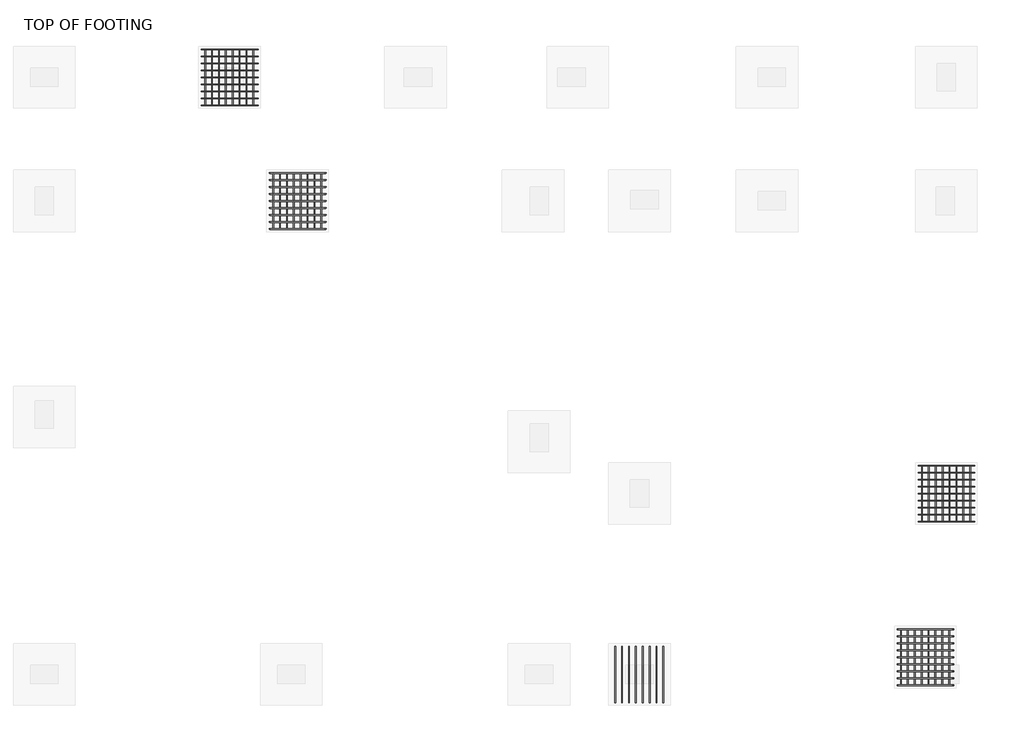
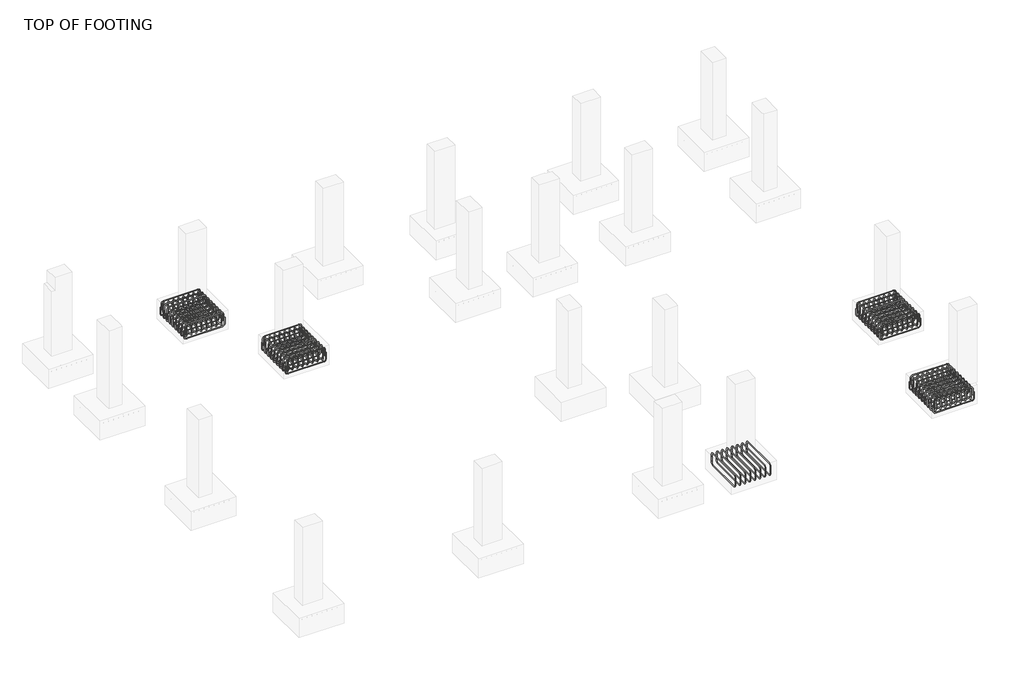
# One storey, part 6 of 20: 18 reinforcing bars.
"""IFC4 building model written with IfcOpenShell, lengths in millimetres."""

from ifc_helpers import new_model, si_unit, point, frame, origin, place, context, project, spatial, polyline, circle_curve, trimmed, segment, composite_curve, source, transform, mapped, element, save
from ifc_brep_helpers import swept_disk

model = new_model("IFC4")

# Units and contexts
model_context = context("Model", 3, world=origin())
ifc_project = project(units=[si_unit("LENGTHUNIT", "METRE", prefix="MILLI")], contexts=[model_context])

# Site, building, storey
site = spatial("IfcSite", under=ifc_project)
building = spatial("IfcBuilding", under=site)
storey = spatial("IfcBuildingStorey", under=building, Name="TOP OF FOOTING", Elevation=-1828.8)

# Reinforcing bars
placement = place(None, origin())
reinforcing_bar_shape = source(origin(), model_context, "Body", "SolidModel", [
    swept_disk(composite_curve([segment(polyline([(8189.02094, -18968.8804373, -2086.1951968), (8189.02094, -18968.8804373, -1938.8951968)]), True, "CONTINUOUS"), segment(trimmed(circle_curve(frame((8189.02094, -19015.2304373, -1938.8951968), z_axis=(1.0, 0.0, 0.0), x_axis=(0.0, 46.35000000000218, 0.0)), 46.35), [point((8189.02094, -18968.8804373, -1938.8951968))], [point((8189.02094, -19015.2304373, -1892.5451968))], True, "CARTESIAN"), True, "CONTINUOUS"), segment(polyline([(8189.02094, -19015.2304373, -1892.5451968), (8189.02094, -19829.8304373, -1892.5451968)]), True, "CONTINUOUS"), segment(trimmed(circle_curve(frame((8189.02094, -19829.8304373, -1938.8951968), z_axis=(1.0, 0.0, 0.0), x_axis=(0.0, 0.0, 46.34999999999991)), 46.35), [point((8189.02094, -19829.8304373, -1892.5451968))], [point((8189.02094, -19876.1804373, -1938.8951968))], True, "CARTESIAN"), True, "CONTINUOUS"), segment(polyline([(8189.02094, -19876.1804373, -1938.8951968), (8189.02094, -19876.1804373, -2086.1951968)]), True, "CONTINUOUS")], self_intersect=False), 6.35),
])
element("IfcReinforcingBar", 1, at=placement, inside=storey, context=model_context, shape_type="MappedRepresentation", body=[
    mapped(reinforcing_bar_shape, transform((0.0, 0.0, 0.0), x_axis=(1.0, 0.0, 0.0), y_axis=(0.0, 1.0, 0.0), z_axis=(0.0, 0.0, 1.0))),
    mapped(reinforcing_bar_shape, transform((-111.2862402, 0.0, 0.0), x_axis=(1.0, 0.0, 0.0), y_axis=(0.0, 1.0, 0.0), z_axis=(0.0, 0.0, 1.0))),
    mapped(reinforcing_bar_shape, transform((-222.5724804, 0.0, 0.0), x_axis=(1.0, 0.0, 0.0), y_axis=(0.0, 1.0, 0.0), z_axis=(0.0, 0.0, 1.0))),
    mapped(reinforcing_bar_shape, transform((-333.8587205, 0.0, 0.0), x_axis=(1.0, 0.0, 0.0), y_axis=(0.0, 1.0, 0.0), z_axis=(0.0, 0.0, 1.0))),
    mapped(reinforcing_bar_shape, transform((-445.1449607, 0.0, 0.0), x_axis=(1.0, 0.0, 0.0), y_axis=(0.0, 1.0, 0.0), z_axis=(0.0, 0.0, 1.0))),
    mapped(reinforcing_bar_shape, transform((-556.4312009, 0.0, 0.0), x_axis=(1.0, 0.0, 0.0), y_axis=(0.0, 1.0, 0.0), z_axis=(0.0, 0.0, 1.0))),
    mapped(reinforcing_bar_shape, transform((-667.7174411, 0.0, 0.0), x_axis=(1.0, 0.0, 0.0), y_axis=(0.0, 1.0, 0.0), z_axis=(0.0, 0.0, 1.0))),
    mapped(reinforcing_bar_shape, transform((-779.0036813, 0.0, 0.0), x_axis=(1.0, 0.0, 0.0), y_axis=(0.0, 1.0, 0.0), z_axis=(0.0, 0.0, 1.0))),
])
reinforcing_bar_2_shape = source(origin(), model_context, "Body", "SolidModel", [
    swept_disk(composite_curve([segment(polyline([(7410.0172587, -18968.8804373, -1979.1645013), (7410.0172587, -18968.8804373, -2126.4645013)]), True, "CONTINUOUS"), segment(trimmed(circle_curve(frame((7410.0172587, -19015.2304373, -2126.4645013), z_axis=(-1.0, 0.0, 0.0), x_axis=(0.0, 46.35000000000218, 0.0)), 46.35), [point((7410.0172587, -18968.8804373, -2126.4645013))], [point((7410.0172587, -19015.2304373, -2172.8145013))], True, "CARTESIAN"), True, "CONTINUOUS"), segment(polyline([(7410.0172587, -19015.2304373, -2172.8145013), (7410.0172587, -19829.8304373, -2172.8145013)]), True, "CONTINUOUS"), segment(trimmed(circle_curve(frame((7410.0172587, -19829.8304373, -2126.4645013), z_axis=(-1.0, 0.0, 0.0), x_axis=(0.0, 0.0, -46.34999999999991)), 46.35), [point((7410.0172587, -19829.8304373, -2172.8145013))], [point((7410.0172587, -19876.1804373, -2126.4645013))], True, "CARTESIAN"), True, "CONTINUOUS"), segment(polyline([(7410.0172587, -19876.1804373, -2126.4645013), (7410.0172587, -19876.1804373, -1979.1645013)]), True, "CONTINUOUS")], self_intersect=False), 6.35),
])
element("IfcReinforcingBar", 2, at=placement, inside=storey, context=model_context, shape_type="MappedRepresentation", body=[
    mapped(reinforcing_bar_2_shape, transform((0.0, 0.0, 0.0), x_axis=(1.0, 0.0, 0.0), y_axis=(0.0, 1.0, 0.0), z_axis=(0.0, 0.0, 1.0))),
    mapped(reinforcing_bar_2_shape, transform((111.2862402, 0.0, 0.0), x_axis=(1.0, 0.0, 0.0), y_axis=(0.0, 1.0, 0.0), z_axis=(0.0, 0.0, 1.0))),
    mapped(reinforcing_bar_2_shape, transform((222.5724804, 0.0, 0.0), x_axis=(1.0, 0.0, 0.0), y_axis=(0.0, 1.0, 0.0), z_axis=(0.0, 0.0, 1.0))),
    mapped(reinforcing_bar_2_shape, transform((333.8587205, 0.0, 0.0), x_axis=(1.0, 0.0, 0.0), y_axis=(0.0, 1.0, 0.0), z_axis=(0.0, 0.0, 1.0))),
    mapped(reinforcing_bar_2_shape, transform((445.1449607, 0.0, 0.0), x_axis=(1.0, 0.0, 0.0), y_axis=(0.0, 1.0, 0.0), z_axis=(0.0, 0.0, 1.0))),
    mapped(reinforcing_bar_2_shape, transform((556.4312009, 0.0, 0.0), x_axis=(1.0, 0.0, 0.0), y_axis=(0.0, 1.0, 0.0), z_axis=(0.0, 0.0, 1.0))),
    mapped(reinforcing_bar_2_shape, transform((667.7174411, 0.0, 0.0), x_axis=(1.0, 0.0, 0.0), y_axis=(0.0, 1.0, 0.0), z_axis=(0.0, 0.0, 1.0))),
    mapped(reinforcing_bar_2_shape, transform((779.0036813, 0.0, 0.0), x_axis=(1.0, 0.0, 0.0), y_axis=(0.0, 1.0, 0.0), z_axis=(0.0, 0.0, 1.0))),
])
reinforcing_bar_3_shape = source(origin(), model_context, "Body", "SolidModel", [
    swept_disk(composite_curve([segment(polyline([(12882.7663908, -18688.8804373, -2006.6587682), (12882.7663908, -18688.8804373, -2153.9587682)]), True, "CONTINUOUS"), segment(trimmed(circle_curve(frame((12836.4163908, -18688.8804373, -2153.9587682), z_axis=(0.0, 1.0, 0.0), x_axis=(46.350000000000364, 0.0, 0.0)), 46.35), [point((12882.7663908, -18688.8804373, -2153.9587682))], [point((12836.4163908, -18688.8804373, -2200.3087682))], True, "CARTESIAN"), True, "CONTINUOUS"), segment(polyline([(12836.4163908, -18688.8804373, -2200.3087682), (12021.8163908, -18688.8804373, -2200.3087682)]), True, "CONTINUOUS"), segment(trimmed(circle_curve(frame((12021.8163908, -18688.8804373, -2153.9587682), z_axis=(0.0, 1.0, 0.0), x_axis=(0.0, 0.0, -46.34999999999991)), 46.35), [point((12021.8163908, -18688.8804373, -2200.3087682))], [point((11975.4663908, -18688.8804373, -2153.9587682))], True, "CARTESIAN"), True, "CONTINUOUS"), segment(polyline([(11975.4663908, -18688.8804373, -2153.9587682), (11975.4663908, -18688.8804373, -2006.6587682)]), True, "CONTINUOUS")], self_intersect=False), 6.35),
])
element("IfcReinforcingBar", 3, at=placement, inside=storey, context=model_context, shape_type="MappedRepresentation", body=[
    mapped(reinforcing_bar_3_shape, transform((0.0, 0.0, 0.0), x_axis=(1.0, 0.0, 0.0), y_axis=(0.0, 1.0, 0.0), z_axis=(0.0, 0.0, 1.0))),
    mapped(reinforcing_bar_3_shape, transform((0.0, -113.4125, 0.0), x_axis=(1.0, 0.0, 0.0), y_axis=(0.0, 1.0, 0.0), z_axis=(0.0, 0.0, 1.0))),
    mapped(reinforcing_bar_3_shape, transform((0.0, -226.825, 0.0), x_axis=(1.0, 0.0, 0.0), y_axis=(0.0, 1.0, 0.0), z_axis=(0.0, 0.0, 1.0))),
    mapped(reinforcing_bar_3_shape, transform((0.0, -340.2375, 0.0), x_axis=(1.0, 0.0, 0.0), y_axis=(0.0, 1.0, 0.0), z_axis=(0.0, 0.0, 1.0))),
    mapped(reinforcing_bar_3_shape, transform((0.0, -453.65, 0.0), x_axis=(1.0, 0.0, 0.0), y_axis=(0.0, 1.0, 0.0), z_axis=(0.0, 0.0, 1.0))),
    mapped(reinforcing_bar_3_shape, transform((0.0, -567.0625, 0.0), x_axis=(1.0, 0.0, 0.0), y_axis=(0.0, 1.0, 0.0), z_axis=(0.0, 0.0, 1.0))),
    mapped(reinforcing_bar_3_shape, transform((0.0, -680.475, 0.0), x_axis=(1.0, 0.0, 0.0), y_axis=(0.0, 1.0, 0.0), z_axis=(0.0, 0.0, 1.0))),
    mapped(reinforcing_bar_3_shape, transform((0.0, -793.8875, 0.0), x_axis=(1.0, 0.0, 0.0), y_axis=(0.0, 1.0, 0.0), z_axis=(0.0, 0.0, 1.0))),
    mapped(reinforcing_bar_3_shape, transform((0.0, -907.3, 0.0), x_axis=(1.0, 0.0, 0.0), y_axis=(0.0, 1.0, 0.0), z_axis=(0.0, 0.0, 1.0))),
])
reinforcing_bar_4_shape = source(origin(), model_context, "Body", "SolidModel", [
    swept_disk(composite_curve([segment(polyline([(11994.9405021, -18688.8804373, -2068.8), (11994.9405021, -18688.8804373, -1921.5)]), True, "CONTINUOUS"), segment(trimmed(circle_curve(frame((12041.2905021, -18688.8804373, -1921.5), z_axis=(0.0, 1.0, 0.0), x_axis=(-46.350000000000364, 0.0, 0.0)), 46.35), [point((11994.9405021, -18688.8804373, -1921.5))], [point((12041.2905021, -18688.8804373, -1875.15))], True, "CARTESIAN"), True, "CONTINUOUS"), segment(polyline([(12041.2905021, -18688.8804373, -1875.15), (12810.7539017, -18688.8804373, -1875.15)]), True, "CONTINUOUS"), segment(trimmed(circle_curve(frame((12810.7539017, -18688.8804373, -1921.5), z_axis=(0.0, 1.0, 0.0), x_axis=(0.0, 0.0, 46.34999999999991)), 46.35), [point((12810.7539017, -18688.8804373, -1875.15))], [point((12857.1039017, -18688.8804373, -1921.5))], True, "CARTESIAN"), True, "CONTINUOUS"), segment(polyline([(12857.1039017, -18688.8804373, -1921.5), (12857.1039017, -18688.8804373, -2068.8)]), True, "CONTINUOUS")], self_intersect=False), 6.35),
])
element("IfcReinforcingBar", 4, at=placement, inside=storey, context=model_context, shape_type="MappedRepresentation", body=[
    mapped(reinforcing_bar_4_shape, transform((0.0, 0.0, 0.0), x_axis=(1.0, 0.0, 0.0), y_axis=(0.0, 1.0, 0.0), z_axis=(0.0, 0.0, 1.0))),
    mapped(reinforcing_bar_4_shape, transform((0.0, -113.4125, 0.0), x_axis=(1.0, 0.0, 0.0), y_axis=(0.0, 1.0, 0.0), z_axis=(0.0, 0.0, 1.0))),
    mapped(reinforcing_bar_4_shape, transform((0.0, -226.825, 0.0), x_axis=(1.0, 0.0, 0.0), y_axis=(0.0, 1.0, 0.0), z_axis=(0.0, 0.0, 1.0))),
    mapped(reinforcing_bar_4_shape, transform((0.0, -340.2375, 0.0), x_axis=(1.0, 0.0, 0.0), y_axis=(0.0, 1.0, 0.0), z_axis=(0.0, 0.0, 1.0))),
    mapped(reinforcing_bar_4_shape, transform((0.0, -453.65, 0.0), x_axis=(1.0, 0.0, 0.0), y_axis=(0.0, 1.0, 0.0), z_axis=(0.0, 0.0, 1.0))),
    mapped(reinforcing_bar_4_shape, transform((0.0, -567.0625, 0.0), x_axis=(1.0, 0.0, 0.0), y_axis=(0.0, 1.0, 0.0), z_axis=(0.0, 0.0, 1.0))),
    mapped(reinforcing_bar_4_shape, transform((0.0, -680.475, 0.0), x_axis=(1.0, 0.0, 0.0), y_axis=(0.0, 1.0, 0.0), z_axis=(0.0, 0.0, 1.0))),
    mapped(reinforcing_bar_4_shape, transform((0.0, -793.8875, 0.0), x_axis=(1.0, 0.0, 0.0), y_axis=(0.0, 1.0, 0.0), z_axis=(0.0, 0.0, 1.0))),
    mapped(reinforcing_bar_4_shape, transform((0.0, -907.3, 0.0), x_axis=(1.0, 0.0, 0.0), y_axis=(0.0, 1.0, 0.0), z_axis=(0.0, 0.0, 1.0))),
])
reinforcing_bar_5_shape = source(origin(), model_context, "Body", "SolidModel", [
    swept_disk(composite_curve([segment(polyline([(12811.2694294, -18688.8804373, -2086.1951968), (12811.2694294, -18688.8804373, -1938.8951968)]), True, "CONTINUOUS"), segment(trimmed(circle_curve(frame((12811.2694294, -18735.2304373, -1938.8951968), z_axis=(1.0, 0.0, 0.0), x_axis=(0.0, 46.35000000000218, 0.0)), 46.35), [point((12811.2694294, -18688.8804373, -1938.8951968))], [point((12811.2694294, -18735.2304373, -1892.5451968))], True, "CARTESIAN"), True, "CONTINUOUS"), segment(polyline([(12811.2694294, -18735.2304373, -1892.5451968), (12811.2694294, -19549.8304373, -1892.5451968)]), True, "CONTINUOUS"), segment(trimmed(circle_curve(frame((12811.2694294, -19549.8304373, -1938.8951968), z_axis=(1.0, 0.0, 0.0), x_axis=(0.0, 0.0, 46.34999999999991)), 46.35), [point((12811.2694294, -19549.8304373, -1892.5451968))], [point((12811.2694294, -19596.1804373, -1938.8951968))], True, "CARTESIAN"), True, "CONTINUOUS"), segment(polyline([(12811.2694294, -19596.1804373, -1938.8951968), (12811.2694294, -19596.1804373, -2086.1951968)]), True, "CONTINUOUS")], self_intersect=False), 6.35),
])
element("IfcReinforcingBar", 5, at=placement, inside=storey, context=model_context, shape_type="MappedRepresentation", body=[
    mapped(reinforcing_bar_5_shape, transform((0.0, 0.0, 0.0), x_axis=(1.0, 0.0, 0.0), y_axis=(0.0, 1.0, 0.0), z_axis=(0.0, 0.0, 1.0))),
    mapped(reinforcing_bar_5_shape, transform((-111.2862402, 0.0, 0.0), x_axis=(1.0, 0.0, 0.0), y_axis=(0.0, 1.0, 0.0), z_axis=(0.0, 0.0, 1.0))),
    mapped(reinforcing_bar_5_shape, transform((-222.5724804, 0.0, 0.0), x_axis=(1.0, 0.0, 0.0), y_axis=(0.0, 1.0, 0.0), z_axis=(0.0, 0.0, 1.0))),
    mapped(reinforcing_bar_5_shape, transform((-333.8587205, 0.0, 0.0), x_axis=(1.0, 0.0, 0.0), y_axis=(0.0, 1.0, 0.0), z_axis=(0.0, 0.0, 1.0))),
    mapped(reinforcing_bar_5_shape, transform((-445.1449607, 0.0, 0.0), x_axis=(1.0, 0.0, 0.0), y_axis=(0.0, 1.0, 0.0), z_axis=(0.0, 0.0, 1.0))),
    mapped(reinforcing_bar_5_shape, transform((-556.4312009, 0.0, 0.0), x_axis=(1.0, 0.0, 0.0), y_axis=(0.0, 1.0, 0.0), z_axis=(0.0, 0.0, 1.0))),
    mapped(reinforcing_bar_5_shape, transform((-667.7174411, 0.0, 0.0), x_axis=(1.0, 0.0, 0.0), y_axis=(0.0, 1.0, 0.0), z_axis=(0.0, 0.0, 1.0))),
    mapped(reinforcing_bar_5_shape, transform((-779.0036813, 0.0, 0.0), x_axis=(1.0, 0.0, 0.0), y_axis=(0.0, 1.0, 0.0), z_axis=(0.0, 0.0, 1.0))),
])
reinforcing_bar_6_shape = source(origin(), model_context, "Body", "SolidModel", [
    swept_disk(composite_curve([segment(polyline([(12032.2657481, -18688.8804373, -1979.1645013), (12032.2657481, -18688.8804373, -2126.4645013)]), True, "CONTINUOUS"), segment(trimmed(circle_curve(frame((12032.2657481, -18735.2304373, -2126.4645013), z_axis=(-1.0, 0.0, 0.0), x_axis=(0.0, 46.35000000000218, 0.0)), 46.35), [point((12032.2657481, -18688.8804373, -2126.4645013))], [point((12032.2657481, -18735.2304373, -2172.8145013))], True, "CARTESIAN"), True, "CONTINUOUS"), segment(polyline([(12032.2657481, -18735.2304373, -2172.8145013), (12032.2657481, -19549.8304373, -2172.8145013)]), True, "CONTINUOUS"), segment(trimmed(circle_curve(frame((12032.2657481, -19549.8304373, -2126.4645013), z_axis=(-1.0, 0.0, 0.0), x_axis=(0.0, 0.0, -46.34999999999991)), 46.35), [point((12032.2657481, -19549.8304373, -2172.8145013))], [point((12032.2657481, -19596.1804373, -2126.4645013))], True, "CARTESIAN"), True, "CONTINUOUS"), segment(polyline([(12032.2657481, -19596.1804373, -2126.4645013), (12032.2657481, -19596.1804373, -1979.1645013)]), True, "CONTINUOUS")], self_intersect=False), 6.35),
])
element("IfcReinforcingBar", 6, at=placement, inside=storey, context=model_context, shape_type="MappedRepresentation", body=[
    mapped(reinforcing_bar_6_shape, transform((0.0, 0.0, 0.0), x_axis=(1.0, 0.0, 0.0), y_axis=(0.0, 1.0, 0.0), z_axis=(0.0, 0.0, 1.0))),
    mapped(reinforcing_bar_6_shape, transform((111.2862402, 0.0, 0.0), x_axis=(1.0, 0.0, 0.0), y_axis=(0.0, 1.0, 0.0), z_axis=(0.0, 0.0, 1.0))),
    mapped(reinforcing_bar_6_shape, transform((222.5724804, 0.0, 0.0), x_axis=(1.0, 0.0, 0.0), y_axis=(0.0, 1.0, 0.0), z_axis=(0.0, 0.0, 1.0))),
    mapped(reinforcing_bar_6_shape, transform((333.8587205, 0.0, 0.0), x_axis=(1.0, 0.0, 0.0), y_axis=(0.0, 1.0, 0.0), z_axis=(0.0, 0.0, 1.0))),
    mapped(reinforcing_bar_6_shape, transform((445.1449607, 0.0, 0.0), x_axis=(1.0, 0.0, 0.0), y_axis=(0.0, 1.0, 0.0), z_axis=(0.0, 0.0, 1.0))),
    mapped(reinforcing_bar_6_shape, transform((556.4312009, 0.0, 0.0), x_axis=(1.0, 0.0, 0.0), y_axis=(0.0, 1.0, 0.0), z_axis=(0.0, 0.0, 1.0))),
    mapped(reinforcing_bar_6_shape, transform((667.7174411, 0.0, 0.0), x_axis=(1.0, 0.0, 0.0), y_axis=(0.0, 1.0, 0.0), z_axis=(0.0, 0.0, 1.0))),
    mapped(reinforcing_bar_6_shape, transform((779.0036813, 0.0, 0.0), x_axis=(1.0, 0.0, 0.0), y_axis=(0.0, 1.0, 0.0), z_axis=(0.0, 0.0, 1.0))),
])
reinforcing_bar_7_shape = source(origin(), model_context, "Body", "SolidModel", [
    swept_disk(composite_curve([segment(polyline([(13222.7663908, -16040.5079597, -2006.6587682), (13222.7663908, -16040.5079597, -2153.9587682)]), True, "CONTINUOUS"), segment(trimmed(circle_curve(frame((13176.4163908, -16040.5079597, -2153.9587682), z_axis=(0.0, 1.0, 0.0), x_axis=(46.350000000000364, 0.0, 0.0)), 46.35), [point((13222.7663908, -16040.5079597, -2153.9587682))], [point((13176.4163908, -16040.5079597, -2200.3087682))], True, "CARTESIAN"), True, "CONTINUOUS"), segment(polyline([(13176.4163908, -16040.5079597, -2200.3087682), (12361.8163908, -16040.5079597, -2200.3087682)]), True, "CONTINUOUS"), segment(trimmed(circle_curve(frame((12361.8163908, -16040.5079597, -2153.9587682), z_axis=(0.0, 1.0, 0.0), x_axis=(0.0, 0.0, -46.34999999999991)), 46.35), [point((12361.8163908, -16040.5079597, -2200.3087682))], [point((12315.4663908, -16040.5079597, -2153.9587682))], True, "CARTESIAN"), True, "CONTINUOUS"), segment(polyline([(12315.4663908, -16040.5079597, -2153.9587682), (12315.4663908, -16040.5079597, -2006.6587682)]), True, "CONTINUOUS")], self_intersect=False), 6.35),
])
element("IfcReinforcingBar", 7, at=placement, inside=storey, context=model_context, shape_type="MappedRepresentation", body=[
    mapped(reinforcing_bar_7_shape, transform((0.0, 0.0, 0.0), x_axis=(1.0, 0.0, 0.0), y_axis=(0.0, 1.0, 0.0), z_axis=(0.0, 0.0, 1.0))),
    mapped(reinforcing_bar_7_shape, transform((0.0, -113.4125, 0.0), x_axis=(1.0, 0.0, 0.0), y_axis=(0.0, 1.0, 0.0), z_axis=(0.0, 0.0, 1.0))),
    mapped(reinforcing_bar_7_shape, transform((0.0, -226.825, 0.0), x_axis=(1.0, 0.0, 0.0), y_axis=(0.0, 1.0, 0.0), z_axis=(0.0, 0.0, 1.0))),
    mapped(reinforcing_bar_7_shape, transform((0.0, -340.2375, 0.0), x_axis=(1.0, 0.0, 0.0), y_axis=(0.0, 1.0, 0.0), z_axis=(0.0, 0.0, 1.0))),
    mapped(reinforcing_bar_7_shape, transform((0.0, -453.65, 0.0), x_axis=(1.0, 0.0, 0.0), y_axis=(0.0, 1.0, 0.0), z_axis=(0.0, 0.0, 1.0))),
    mapped(reinforcing_bar_7_shape, transform((0.0, -567.0625, 0.0), x_axis=(1.0, 0.0, 0.0), y_axis=(0.0, 1.0, 0.0), z_axis=(0.0, 0.0, 1.0))),
    mapped(reinforcing_bar_7_shape, transform((0.0, -680.475, 0.0), x_axis=(1.0, 0.0, 0.0), y_axis=(0.0, 1.0, 0.0), z_axis=(0.0, 0.0, 1.0))),
    mapped(reinforcing_bar_7_shape, transform((0.0, -793.8875, 0.0), x_axis=(1.0, 0.0, 0.0), y_axis=(0.0, 1.0, 0.0), z_axis=(0.0, 0.0, 1.0))),
    mapped(reinforcing_bar_7_shape, transform((0.0, -907.3, 0.0), x_axis=(1.0, 0.0, 0.0), y_axis=(0.0, 1.0, 0.0), z_axis=(0.0, 0.0, 1.0))),
])
reinforcing_bar_8_shape = source(origin(), model_context, "Body", "SolidModel", [
    swept_disk(composite_curve([segment(polyline([(12334.9405021, -16040.5079597, -2068.8), (12334.9405021, -16040.5079597, -1921.5)]), True, "CONTINUOUS"), segment(trimmed(circle_curve(frame((12381.2905021, -16040.5079597, -1921.5), z_axis=(0.0, 1.0, 0.0), x_axis=(-46.350000000000364, 0.0, 0.0)), 46.35), [point((12334.9405021, -16040.5079597, -1921.5))], [point((12381.2905021, -16040.5079597, -1875.15))], True, "CARTESIAN"), True, "CONTINUOUS"), segment(polyline([(12381.2905021, -16040.5079597, -1875.15), (13150.7539017, -16040.5079597, -1875.15)]), True, "CONTINUOUS"), segment(trimmed(circle_curve(frame((13150.7539017, -16040.5079597, -1921.5), z_axis=(0.0, 1.0, 0.0), x_axis=(0.0, 0.0, 46.34999999999991)), 46.35), [point((13150.7539017, -16040.5079597, -1875.15))], [point((13197.1039017, -16040.5079597, -1921.5))], True, "CARTESIAN"), True, "CONTINUOUS"), segment(polyline([(13197.1039017, -16040.5079597, -1921.5), (13197.1039017, -16040.5079597, -2068.8)]), True, "CONTINUOUS")], self_intersect=False), 6.35),
])
element("IfcReinforcingBar", 8, at=placement, inside=storey, context=model_context, shape_type="MappedRepresentation", body=[
    mapped(reinforcing_bar_8_shape, transform((0.0, 0.0, 0.0), x_axis=(1.0, 0.0, 0.0), y_axis=(0.0, 1.0, 0.0), z_axis=(0.0, 0.0, 1.0))),
    mapped(reinforcing_bar_8_shape, transform((0.0, -113.4125, 0.0), x_axis=(1.0, 0.0, 0.0), y_axis=(0.0, 1.0, 0.0), z_axis=(0.0, 0.0, 1.0))),
    mapped(reinforcing_bar_8_shape, transform((0.0, -226.825, 0.0), x_axis=(1.0, 0.0, 0.0), y_axis=(0.0, 1.0, 0.0), z_axis=(0.0, 0.0, 1.0))),
    mapped(reinforcing_bar_8_shape, transform((0.0, -340.2375, 0.0), x_axis=(1.0, 0.0, 0.0), y_axis=(0.0, 1.0, 0.0), z_axis=(0.0, 0.0, 1.0))),
    mapped(reinforcing_bar_8_shape, transform((0.0, -453.65, 0.0), x_axis=(1.0, 0.0, 0.0), y_axis=(0.0, 1.0, 0.0), z_axis=(0.0, 0.0, 1.0))),
    mapped(reinforcing_bar_8_shape, transform((0.0, -567.0625, 0.0), x_axis=(1.0, 0.0, 0.0), y_axis=(0.0, 1.0, 0.0), z_axis=(0.0, 0.0, 1.0))),
    mapped(reinforcing_bar_8_shape, transform((0.0, -680.475, 0.0), x_axis=(1.0, 0.0, 0.0), y_axis=(0.0, 1.0, 0.0), z_axis=(0.0, 0.0, 1.0))),
    mapped(reinforcing_bar_8_shape, transform((0.0, -793.8875, 0.0), x_axis=(1.0, 0.0, 0.0), y_axis=(0.0, 1.0, 0.0), z_axis=(0.0, 0.0, 1.0))),
    mapped(reinforcing_bar_8_shape, transform((0.0, -907.3, 0.0), x_axis=(1.0, 0.0, 0.0), y_axis=(0.0, 1.0, 0.0), z_axis=(0.0, 0.0, 1.0))),
])
reinforcing_bar_9_shape = source(origin(), model_context, "Body", "SolidModel", [
    swept_disk(composite_curve([segment(polyline([(13151.2694294, -16040.5079597, -2086.1951968), (13151.2694294, -16040.5079597, -1938.8951968)]), True, "CONTINUOUS"), segment(trimmed(circle_curve(frame((13151.2694294, -16086.8579597, -1938.8951968), z_axis=(1.0, 0.0, 0.0), x_axis=(0.0, 46.350000000000364, 0.0)), 46.35), [point((13151.2694294, -16040.5079597, -1938.8951968))], [point((13151.2694294, -16086.8579597, -1892.5451968))], True, "CARTESIAN"), True, "CONTINUOUS"), segment(polyline([(13151.2694294, -16086.8579597, -1892.5451968), (13151.2694294, -16901.4579597, -1892.5451968)]), True, "CONTINUOUS"), segment(trimmed(circle_curve(frame((13151.2694294, -16901.4579597, -1938.8951968), z_axis=(1.0, 0.0, 0.0), x_axis=(0.0, 0.0, 46.34999999999991)), 46.35), [point((13151.2694294, -16901.4579597, -1892.5451968))], [point((13151.2694294, -16947.8079597, -1938.8951968))], True, "CARTESIAN"), True, "CONTINUOUS"), segment(polyline([(13151.2694294, -16947.8079597, -1938.8951968), (13151.2694294, -16947.8079597, -2086.1951968)]), True, "CONTINUOUS")], self_intersect=False), 6.35),
])
element("IfcReinforcingBar", 9, at=placement, inside=storey, context=model_context, shape_type="MappedRepresentation", body=[
    mapped(reinforcing_bar_9_shape, transform((0.0, 0.0, 0.0), x_axis=(1.0, 0.0, 0.0), y_axis=(0.0, 1.0, 0.0), z_axis=(0.0, 0.0, 1.0))),
    mapped(reinforcing_bar_9_shape, transform((-111.2862402, 0.0, 0.0), x_axis=(1.0, 0.0, 0.0), y_axis=(0.0, 1.0, 0.0), z_axis=(0.0, 0.0, 1.0))),
    mapped(reinforcing_bar_9_shape, transform((-222.5724804, 0.0, 0.0), x_axis=(1.0, 0.0, 0.0), y_axis=(0.0, 1.0, 0.0), z_axis=(0.0, 0.0, 1.0))),
    mapped(reinforcing_bar_9_shape, transform((-333.8587205, 0.0, 0.0), x_axis=(1.0, 0.0, 0.0), y_axis=(0.0, 1.0, 0.0), z_axis=(0.0, 0.0, 1.0))),
    mapped(reinforcing_bar_9_shape, transform((-445.1449607, 0.0, 0.0), x_axis=(1.0, 0.0, 0.0), y_axis=(0.0, 1.0, 0.0), z_axis=(0.0, 0.0, 1.0))),
    mapped(reinforcing_bar_9_shape, transform((-556.4312009, 0.0, 0.0), x_axis=(1.0, 0.0, 0.0), y_axis=(0.0, 1.0, 0.0), z_axis=(0.0, 0.0, 1.0))),
    mapped(reinforcing_bar_9_shape, transform((-667.7174411, 0.0, 0.0), x_axis=(1.0, 0.0, 0.0), y_axis=(0.0, 1.0, 0.0), z_axis=(0.0, 0.0, 1.0))),
    mapped(reinforcing_bar_9_shape, transform((-779.0036813, 0.0, 0.0), x_axis=(1.0, 0.0, 0.0), y_axis=(0.0, 1.0, 0.0), z_axis=(0.0, 0.0, 1.0))),
])
reinforcing_bar_10_shape = source(origin(), model_context, "Body", "SolidModel", [
    swept_disk(composite_curve([segment(polyline([(12372.2657481, -16040.5079597, -1979.1645013), (12372.2657481, -16040.5079597, -2126.4645013)]), True, "CONTINUOUS"), segment(trimmed(circle_curve(frame((12372.2657481, -16086.8579597, -2126.4645013), z_axis=(-1.0, 0.0, 0.0), x_axis=(0.0, 46.350000000000364, 0.0)), 46.35), [point((12372.2657481, -16040.5079597, -2126.4645013))], [point((12372.2657481, -16086.8579597, -2172.8145013))], True, "CARTESIAN"), True, "CONTINUOUS"), segment(polyline([(12372.2657481, -16086.8579597, -2172.8145013), (12372.2657481, -16901.4579597, -2172.8145013)]), True, "CONTINUOUS"), segment(trimmed(circle_curve(frame((12372.2657481, -16901.4579597, -2126.4645013), z_axis=(-1.0, 0.0, 0.0), x_axis=(0.0, 0.0, -46.34999999999991)), 46.35), [point((12372.2657481, -16901.4579597, -2172.8145013))], [point((12372.2657481, -16947.8079597, -2126.4645013))], True, "CARTESIAN"), True, "CONTINUOUS"), segment(polyline([(12372.2657481, -16947.8079597, -2126.4645013), (12372.2657481, -16947.8079597, -1979.1645013)]), True, "CONTINUOUS")], self_intersect=False), 6.35),
])
element("IfcReinforcingBar", 10, at=placement, inside=storey, context=model_context, shape_type="MappedRepresentation", body=[
    mapped(reinforcing_bar_10_shape, transform((0.0, 0.0, 0.0), x_axis=(1.0, 0.0, 0.0), y_axis=(0.0, 1.0, 0.0), z_axis=(0.0, 0.0, 1.0))),
    mapped(reinforcing_bar_10_shape, transform((111.2862402, 0.0, 0.0), x_axis=(1.0, 0.0, 0.0), y_axis=(0.0, 1.0, 0.0), z_axis=(0.0, 0.0, 1.0))),
    mapped(reinforcing_bar_10_shape, transform((222.5724804, 0.0, 0.0), x_axis=(1.0, 0.0, 0.0), y_axis=(0.0, 1.0, 0.0), z_axis=(0.0, 0.0, 1.0))),
    mapped(reinforcing_bar_10_shape, transform((333.8587205, 0.0, 0.0), x_axis=(1.0, 0.0, 0.0), y_axis=(0.0, 1.0, 0.0), z_axis=(0.0, 0.0, 1.0))),
    mapped(reinforcing_bar_10_shape, transform((445.1449607, 0.0, 0.0), x_axis=(1.0, 0.0, 0.0), y_axis=(0.0, 1.0, 0.0), z_axis=(0.0, 0.0, 1.0))),
    mapped(reinforcing_bar_10_shape, transform((556.4312009, 0.0, 0.0), x_axis=(1.0, 0.0, 0.0), y_axis=(0.0, 1.0, 0.0), z_axis=(0.0, 0.0, 1.0))),
    mapped(reinforcing_bar_10_shape, transform((667.7174411, 0.0, 0.0), x_axis=(1.0, 0.0, 0.0), y_axis=(0.0, 1.0, 0.0), z_axis=(0.0, 0.0, 1.0))),
    mapped(reinforcing_bar_10_shape, transform((779.0036813, 0.0, 0.0), x_axis=(1.0, 0.0, 0.0), y_axis=(0.0, 1.0, 0.0), z_axis=(0.0, 0.0, 1.0))),
])
reinforcing_bar_11_shape = source(origin(), model_context, "Body", "SolidModel", [
    swept_disk(composite_curve([segment(polyline([(1628.3796816, -9303.4578267, -2006.6587682), (1628.3796816, -9303.4578267, -2153.9587682)]), True, "CONTINUOUS"), segment(trimmed(circle_curve(frame((1582.0296816, -9303.4578267, -2153.9587682), z_axis=(0.0, 1.0, 0.0), x_axis=(46.34999999999991, 0.0, 0.0)), 46.35), [point((1628.3796816, -9303.4578267, -2153.9587682))], [point((1582.0296816, -9303.4578267, -2200.3087682))], True, "CARTESIAN"), True, "CONTINUOUS"), segment(polyline([(1582.0296816, -9303.4578267, -2200.3087682), (767.4296816, -9303.4578267, -2200.3087682)]), True, "CONTINUOUS"), segment(trimmed(circle_curve(frame((767.4296816, -9303.4578267, -2153.9587682), z_axis=(0.0, 1.0, 0.0), x_axis=(0.0, 0.0, -46.34999999999991)), 46.35), [point((767.4296816, -9303.4578267, -2200.3087682))], [point((721.0796816, -9303.4578267, -2153.9587682))], True, "CARTESIAN"), True, "CONTINUOUS"), segment(polyline([(721.0796816, -9303.4578267, -2153.9587682), (721.0796816, -9303.4578267, -2006.6587682)]), True, "CONTINUOUS")], self_intersect=False), 6.35),
])
element("IfcReinforcingBar", 11, at=placement, inside=storey, context=model_context, shape_type="MappedRepresentation", body=[
    mapped(reinforcing_bar_11_shape, transform((0.0, 0.0, 0.0), x_axis=(1.0, 0.0, 0.0), y_axis=(0.0, 1.0, 0.0), z_axis=(0.0, 0.0, 1.0))),
    mapped(reinforcing_bar_11_shape, transform((0.0, -113.4125, 0.0), x_axis=(1.0, 0.0, 0.0), y_axis=(0.0, 1.0, 0.0), z_axis=(0.0, 0.0, 1.0))),
    mapped(reinforcing_bar_11_shape, transform((0.0, -226.825, 0.0), x_axis=(1.0, 0.0, 0.0), y_axis=(0.0, 1.0, 0.0), z_axis=(0.0, 0.0, 1.0))),
    mapped(reinforcing_bar_11_shape, transform((0.0, -340.2375, 0.0), x_axis=(1.0, 0.0, 0.0), y_axis=(0.0, 1.0, 0.0), z_axis=(0.0, 0.0, 1.0))),
    mapped(reinforcing_bar_11_shape, transform((0.0, -453.65, 0.0), x_axis=(1.0, 0.0, 0.0), y_axis=(0.0, 1.0, 0.0), z_axis=(0.0, 0.0, 1.0))),
    mapped(reinforcing_bar_11_shape, transform((0.0, -567.0625, 0.0), x_axis=(1.0, 0.0, 0.0), y_axis=(0.0, 1.0, 0.0), z_axis=(0.0, 0.0, 1.0))),
    mapped(reinforcing_bar_11_shape, transform((0.0, -680.475, 0.0), x_axis=(1.0, 0.0, 0.0), y_axis=(0.0, 1.0, 0.0), z_axis=(0.0, 0.0, 1.0))),
    mapped(reinforcing_bar_11_shape, transform((0.0, -793.8875, 0.0), x_axis=(1.0, 0.0, 0.0), y_axis=(0.0, 1.0, 0.0), z_axis=(0.0, 0.0, 1.0))),
    mapped(reinforcing_bar_11_shape, transform((0.0, -907.3, 0.0), x_axis=(1.0, 0.0, 0.0), y_axis=(0.0, 1.0, 0.0), z_axis=(0.0, 0.0, 1.0))),
])
reinforcing_bar_12_shape = source(origin(), model_context, "Body", "SolidModel", [
    swept_disk(composite_curve([segment(polyline([(740.553793, -9303.4578267, -2068.8), (740.553793, -9303.4578267, -1921.5)]), True, "CONTINUOUS"), segment(trimmed(circle_curve(frame((786.903793, -9303.4578267, -1921.5), z_axis=(0.0, 1.0, 0.0), x_axis=(-46.34999999999991, 0.0, 0.0)), 46.35), [point((740.553793, -9303.4578267, -1921.5))], [point((786.903793, -9303.4578267, -1875.15))], True, "CARTESIAN"), True, "CONTINUOUS"), segment(polyline([(786.903793, -9303.4578267, -1875.15), (1556.3671926, -9303.4578267, -1875.15)]), True, "CONTINUOUS"), segment(trimmed(circle_curve(frame((1556.3671926, -9303.4578267, -1921.5), z_axis=(0.0, 1.0, 0.0), x_axis=(0.0, 0.0, 46.34999999999991)), 46.35), [point((1556.3671926, -9303.4578267, -1875.15))], [point((1602.7171926, -9303.4578267, -1921.5))], True, "CARTESIAN"), True, "CONTINUOUS"), segment(polyline([(1602.7171926, -9303.4578267, -1921.5), (1602.7171926, -9303.4578267, -2068.8)]), True, "CONTINUOUS")], self_intersect=False), 6.35),
])
element("IfcReinforcingBar", 12, at=placement, inside=storey, context=model_context, shape_type="MappedRepresentation", body=[
    mapped(reinforcing_bar_12_shape, transform((0.0, 0.0, 0.0), x_axis=(1.0, 0.0, 0.0), y_axis=(0.0, 1.0, 0.0), z_axis=(0.0, 0.0, 1.0))),
    mapped(reinforcing_bar_12_shape, transform((0.0, -113.4125, 0.0), x_axis=(1.0, 0.0, 0.0), y_axis=(0.0, 1.0, 0.0), z_axis=(0.0, 0.0, 1.0))),
    mapped(reinforcing_bar_12_shape, transform((0.0, -226.825, 0.0), x_axis=(1.0, 0.0, 0.0), y_axis=(0.0, 1.0, 0.0), z_axis=(0.0, 0.0, 1.0))),
    mapped(reinforcing_bar_12_shape, transform((0.0, -340.2375, 0.0), x_axis=(1.0, 0.0, 0.0), y_axis=(0.0, 1.0, 0.0), z_axis=(0.0, 0.0, 1.0))),
    mapped(reinforcing_bar_12_shape, transform((0.0, -453.65, 0.0), x_axis=(1.0, 0.0, 0.0), y_axis=(0.0, 1.0, 0.0), z_axis=(0.0, 0.0, 1.0))),
    mapped(reinforcing_bar_12_shape, transform((0.0, -567.0625, 0.0), x_axis=(1.0, 0.0, 0.0), y_axis=(0.0, 1.0, 0.0), z_axis=(0.0, 0.0, 1.0))),
    mapped(reinforcing_bar_12_shape, transform((0.0, -680.475, 0.0), x_axis=(1.0, 0.0, 0.0), y_axis=(0.0, 1.0, 0.0), z_axis=(0.0, 0.0, 1.0))),
    mapped(reinforcing_bar_12_shape, transform((0.0, -793.8875, 0.0), x_axis=(1.0, 0.0, 0.0), y_axis=(0.0, 1.0, 0.0), z_axis=(0.0, 0.0, 1.0))),
    mapped(reinforcing_bar_12_shape, transform((0.0, -907.3, 0.0), x_axis=(1.0, 0.0, 0.0), y_axis=(0.0, 1.0, 0.0), z_axis=(0.0, 0.0, 1.0))),
])
reinforcing_bar_13_shape = source(origin(), model_context, "Body", "SolidModel", [
    swept_disk(composite_curve([segment(polyline([(1556.8827202, -9303.4578267, -2086.1951968), (1556.8827202, -9303.4578267, -1938.8951968)]), True, "CONTINUOUS"), segment(trimmed(circle_curve(frame((1556.8827202, -9349.8078267, -1938.8951968), z_axis=(1.0, 0.0, 0.0), x_axis=(0.0, 46.350000000000364, 0.0)), 46.35), [point((1556.8827202, -9303.4578267, -1938.8951968))], [point((1556.8827202, -9349.8078267, -1892.5451968))], True, "CARTESIAN"), True, "CONTINUOUS"), segment(polyline([(1556.8827202, -9349.8078267, -1892.5451968), (1556.8827202, -10164.4078267, -1892.5451968)]), True, "CONTINUOUS"), segment(trimmed(circle_curve(frame((1556.8827202, -10164.4078267, -1938.8951968), z_axis=(1.0, 0.0, 0.0), x_axis=(0.0, 0.0, 46.34999999999991)), 46.35), [point((1556.8827202, -10164.4078267, -1892.5451968))], [point((1556.8827202, -10210.7578267, -1938.8951968))], True, "CARTESIAN"), True, "CONTINUOUS"), segment(polyline([(1556.8827202, -10210.7578267, -1938.8951968), (1556.8827202, -10210.7578267, -2086.1951968)]), True, "CONTINUOUS")], self_intersect=False), 6.35),
])
element("IfcReinforcingBar", 13, at=placement, inside=storey, context=model_context, shape_type="MappedRepresentation", body=[
    mapped(reinforcing_bar_13_shape, transform((0.0, 0.0, 0.0), x_axis=(1.0, 0.0, 0.0), y_axis=(0.0, 1.0, 0.0), z_axis=(0.0, 0.0, 1.0))),
    mapped(reinforcing_bar_13_shape, transform((-111.2862402, 0.0, 0.0), x_axis=(1.0, 0.0, 0.0), y_axis=(0.0, 1.0, 0.0), z_axis=(0.0, 0.0, 1.0))),
    mapped(reinforcing_bar_13_shape, transform((-222.5724804, 0.0, 0.0), x_axis=(1.0, 0.0, 0.0), y_axis=(0.0, 1.0, 0.0), z_axis=(0.0, 0.0, 1.0))),
    mapped(reinforcing_bar_13_shape, transform((-333.8587205, 0.0, 0.0), x_axis=(1.0, 0.0, 0.0), y_axis=(0.0, 1.0, 0.0), z_axis=(0.0, 0.0, 1.0))),
    mapped(reinforcing_bar_13_shape, transform((-445.1449607, 0.0, 0.0), x_axis=(1.0, 0.0, 0.0), y_axis=(0.0, 1.0, 0.0), z_axis=(0.0, 0.0, 1.0))),
    mapped(reinforcing_bar_13_shape, transform((-556.4312009, 0.0, 0.0), x_axis=(1.0, 0.0, 0.0), y_axis=(0.0, 1.0, 0.0), z_axis=(0.0, 0.0, 1.0))),
    mapped(reinforcing_bar_13_shape, transform((-667.7174411, 0.0, 0.0), x_axis=(1.0, 0.0, 0.0), y_axis=(0.0, 1.0, 0.0), z_axis=(0.0, 0.0, 1.0))),
    mapped(reinforcing_bar_13_shape, transform((-779.0036813, 0.0, 0.0), x_axis=(1.0, 0.0, 0.0), y_axis=(0.0, 1.0, 0.0), z_axis=(0.0, 0.0, 1.0))),
])
reinforcing_bar_14_shape = source(origin(), model_context, "Body", "SolidModel", [
    swept_disk(composite_curve([segment(polyline([(777.879039, -9303.4578267, -1979.1645013), (777.879039, -9303.4578267, -2126.4645013)]), True, "CONTINUOUS"), segment(trimmed(circle_curve(frame((777.879039, -9349.8078267, -2126.4645013), z_axis=(-1.0, 0.0, 0.0), x_axis=(0.0, 46.350000000000364, 0.0)), 46.35), [point((777.879039, -9303.4578267, -2126.4645013))], [point((777.879039, -9349.8078267, -2172.8145013))], True, "CARTESIAN"), True, "CONTINUOUS"), segment(polyline([(777.879039, -9349.8078267, -2172.8145013), (777.879039, -10164.4078267, -2172.8145013)]), True, "CONTINUOUS"), segment(trimmed(circle_curve(frame((777.879039, -10164.4078267, -2126.4645013), z_axis=(-1.0, 0.0, 0.0), x_axis=(0.0, 0.0, -46.34999999999991)), 46.35), [point((777.879039, -10164.4078267, -2172.8145013))], [point((777.879039, -10210.7578267, -2126.4645013))], True, "CARTESIAN"), True, "CONTINUOUS"), segment(polyline([(777.879039, -10210.7578267, -2126.4645013), (777.879039, -10210.7578267, -1979.1645013)]), True, "CONTINUOUS")], self_intersect=False), 6.35),
])
element("IfcReinforcingBar", 14, at=placement, inside=storey, context=model_context, shape_type="MappedRepresentation", body=[
    mapped(reinforcing_bar_14_shape, transform((0.0, 0.0, 0.0), x_axis=(1.0, 0.0, 0.0), y_axis=(0.0, 1.0, 0.0), z_axis=(0.0, 0.0, 1.0))),
    mapped(reinforcing_bar_14_shape, transform((111.2862402, 0.0, 0.0), x_axis=(1.0, 0.0, 0.0), y_axis=(0.0, 1.0, 0.0), z_axis=(0.0, 0.0, 1.0))),
    mapped(reinforcing_bar_14_shape, transform((222.5724804, 0.0, 0.0), x_axis=(1.0, 0.0, 0.0), y_axis=(0.0, 1.0, 0.0), z_axis=(0.0, 0.0, 1.0))),
    mapped(reinforcing_bar_14_shape, transform((333.8587205, 0.0, 0.0), x_axis=(1.0, 0.0, 0.0), y_axis=(0.0, 1.0, 0.0), z_axis=(0.0, 0.0, 1.0))),
    mapped(reinforcing_bar_14_shape, transform((445.1449607, 0.0, 0.0), x_axis=(1.0, 0.0, 0.0), y_axis=(0.0, 1.0, 0.0), z_axis=(0.0, 0.0, 1.0))),
    mapped(reinforcing_bar_14_shape, transform((556.4312009, 0.0, 0.0), x_axis=(1.0, 0.0, 0.0), y_axis=(0.0, 1.0, 0.0), z_axis=(0.0, 0.0, 1.0))),
    mapped(reinforcing_bar_14_shape, transform((667.7174411, 0.0, 0.0), x_axis=(1.0, 0.0, 0.0), y_axis=(0.0, 1.0, 0.0), z_axis=(0.0, 0.0, 1.0))),
    mapped(reinforcing_bar_14_shape, transform((779.0036813, 0.0, 0.0), x_axis=(1.0, 0.0, 0.0), y_axis=(0.0, 1.0, 0.0), z_axis=(0.0, 0.0, 1.0))),
])
reinforcing_bar_15_shape = source(origin(), model_context, "Body", "SolidModel", [
    swept_disk(composite_curve([segment(polyline([(2728.3796816, -11304.2470059, -2006.6587682), (2728.3796816, -11304.2470059, -2153.9587682)]), True, "CONTINUOUS"), segment(trimmed(circle_curve(frame((2682.0296816, -11304.2470059, -2153.9587682), z_axis=(0.0, 1.0, 0.0), x_axis=(46.34999999999991, 0.0, 0.0)), 46.35), [point((2728.3796816, -11304.2470059, -2153.9587682))], [point((2682.0296816, -11304.2470059, -2200.3087682))], True, "CARTESIAN"), True, "CONTINUOUS"), segment(polyline([(2682.0296816, -11304.2470059, -2200.3087682), (1867.4296816, -11304.2470059, -2200.3087682)]), True, "CONTINUOUS"), segment(trimmed(circle_curve(frame((1867.4296816, -11304.2470059, -2153.9587682), z_axis=(0.0, 1.0, 0.0), x_axis=(0.0, 0.0, -46.34999999999991)), 46.35), [point((1867.4296816, -11304.2470059, -2200.3087682))], [point((1821.0796816, -11304.2470059, -2153.9587682))], True, "CARTESIAN"), True, "CONTINUOUS"), segment(polyline([(1821.0796816, -11304.2470059, -2153.9587682), (1821.0796816, -11304.2470059, -2006.6587682)]), True, "CONTINUOUS")], self_intersect=False), 6.35),
])
element("IfcReinforcingBar", 15, at=placement, inside=storey, context=model_context, shape_type="MappedRepresentation", body=[
    mapped(reinforcing_bar_15_shape, transform((0.0, 0.0, 0.0), x_axis=(1.0, 0.0, 0.0), y_axis=(0.0, 1.0, 0.0), z_axis=(0.0, 0.0, 1.0))),
    mapped(reinforcing_bar_15_shape, transform((0.0, -113.4125, 0.0), x_axis=(1.0, 0.0, 0.0), y_axis=(0.0, 1.0, 0.0), z_axis=(0.0, 0.0, 1.0))),
    mapped(reinforcing_bar_15_shape, transform((0.0, -226.825, 0.0), x_axis=(1.0, 0.0, 0.0), y_axis=(0.0, 1.0, 0.0), z_axis=(0.0, 0.0, 1.0))),
    mapped(reinforcing_bar_15_shape, transform((0.0, -340.2375, 0.0), x_axis=(1.0, 0.0, 0.0), y_axis=(0.0, 1.0, 0.0), z_axis=(0.0, 0.0, 1.0))),
    mapped(reinforcing_bar_15_shape, transform((0.0, -453.65, 0.0), x_axis=(1.0, 0.0, 0.0), y_axis=(0.0, 1.0, 0.0), z_axis=(0.0, 0.0, 1.0))),
    mapped(reinforcing_bar_15_shape, transform((0.0, -567.0625, 0.0), x_axis=(1.0, 0.0, 0.0), y_axis=(0.0, 1.0, 0.0), z_axis=(0.0, 0.0, 1.0))),
    mapped(reinforcing_bar_15_shape, transform((0.0, -680.475, 0.0), x_axis=(1.0, 0.0, 0.0), y_axis=(0.0, 1.0, 0.0), z_axis=(0.0, 0.0, 1.0))),
    mapped(reinforcing_bar_15_shape, transform((0.0, -793.8875, 0.0), x_axis=(1.0, 0.0, 0.0), y_axis=(0.0, 1.0, 0.0), z_axis=(0.0, 0.0, 1.0))),
    mapped(reinforcing_bar_15_shape, transform((0.0, -907.3, 0.0), x_axis=(1.0, 0.0, 0.0), y_axis=(0.0, 1.0, 0.0), z_axis=(0.0, 0.0, 1.0))),
])
reinforcing_bar_16_shape = source(origin(), model_context, "Body", "SolidModel", [
    swept_disk(composite_curve([segment(polyline([(1840.553793, -11304.2470059, -2068.8), (1840.553793, -11304.2470059, -1921.5)]), True, "CONTINUOUS"), segment(trimmed(circle_curve(frame((1886.903793, -11304.2470059, -1921.5), z_axis=(0.0, 1.0, 0.0), x_axis=(-46.34999999999991, 0.0, 0.0)), 46.35), [point((1840.553793, -11304.2470059, -1921.5))], [point((1886.903793, -11304.2470059, -1875.15))], True, "CARTESIAN"), True, "CONTINUOUS"), segment(polyline([(1886.903793, -11304.2470059, -1875.15), (2656.3671926, -11304.2470059, -1875.15)]), True, "CONTINUOUS"), segment(trimmed(circle_curve(frame((2656.3671926, -11304.2470059, -1921.5), z_axis=(0.0, 1.0, 0.0), x_axis=(0.0, 0.0, 46.34999999999991)), 46.35), [point((2656.3671926, -11304.2470059, -1875.15))], [point((2702.7171926, -11304.2470059, -1921.5))], True, "CARTESIAN"), True, "CONTINUOUS"), segment(polyline([(2702.7171926, -11304.2470059, -1921.5), (2702.7171926, -11304.2470059, -2068.8)]), True, "CONTINUOUS")], self_intersect=False), 6.35),
])
element("IfcReinforcingBar", 16, at=placement, inside=storey, context=model_context, shape_type="MappedRepresentation", body=[
    mapped(reinforcing_bar_16_shape, transform((0.0, 0.0, 0.0), x_axis=(1.0, 0.0, 0.0), y_axis=(0.0, 1.0, 0.0), z_axis=(0.0, 0.0, 1.0))),
    mapped(reinforcing_bar_16_shape, transform((0.0, -113.4125, 0.0), x_axis=(1.0, 0.0, 0.0), y_axis=(0.0, 1.0, 0.0), z_axis=(0.0, 0.0, 1.0))),
    mapped(reinforcing_bar_16_shape, transform((0.0, -226.825, 0.0), x_axis=(1.0, 0.0, 0.0), y_axis=(0.0, 1.0, 0.0), z_axis=(0.0, 0.0, 1.0))),
    mapped(reinforcing_bar_16_shape, transform((0.0, -340.2375, 0.0), x_axis=(1.0, 0.0, 0.0), y_axis=(0.0, 1.0, 0.0), z_axis=(0.0, 0.0, 1.0))),
    mapped(reinforcing_bar_16_shape, transform((0.0, -453.65, 0.0), x_axis=(1.0, 0.0, 0.0), y_axis=(0.0, 1.0, 0.0), z_axis=(0.0, 0.0, 1.0))),
    mapped(reinforcing_bar_16_shape, transform((0.0, -567.0625, 0.0), x_axis=(1.0, 0.0, 0.0), y_axis=(0.0, 1.0, 0.0), z_axis=(0.0, 0.0, 1.0))),
    mapped(reinforcing_bar_16_shape, transform((0.0, -680.475, 0.0), x_axis=(1.0, 0.0, 0.0), y_axis=(0.0, 1.0, 0.0), z_axis=(0.0, 0.0, 1.0))),
    mapped(reinforcing_bar_16_shape, transform((0.0, -793.8875, 0.0), x_axis=(1.0, 0.0, 0.0), y_axis=(0.0, 1.0, 0.0), z_axis=(0.0, 0.0, 1.0))),
    mapped(reinforcing_bar_16_shape, transform((0.0, -907.3, 0.0), x_axis=(1.0, 0.0, 0.0), y_axis=(0.0, 1.0, 0.0), z_axis=(0.0, 0.0, 1.0))),
])
reinforcing_bar_17_shape = source(origin(), model_context, "Body", "SolidModel", [
    swept_disk(composite_curve([segment(polyline([(2656.8827202, -11304.2470059, -2086.1951968), (2656.8827202, -11304.2470059, -1938.8951968)]), True, "CONTINUOUS"), segment(trimmed(circle_curve(frame((2656.8827202, -11350.5970059, -1938.8951968), z_axis=(1.0, 0.0, 0.0), x_axis=(0.0, 46.349999999998545, 0.0)), 46.35), [point((2656.8827202, -11304.2470059, -1938.8951968))], [point((2656.8827202, -11350.5970059, -1892.5451968))], True, "CARTESIAN"), True, "CONTINUOUS"), segment(polyline([(2656.8827202, -11350.5970059, -1892.5451968), (2656.8827202, -12165.1970059, -1892.5451968)]), True, "CONTINUOUS"), segment(trimmed(circle_curve(frame((2656.8827202, -12165.1970059, -1938.8951968), z_axis=(1.0, 0.0, 0.0), x_axis=(0.0, 0.0, 46.34999999999991)), 46.35), [point((2656.8827202, -12165.1970059, -1892.5451968))], [point((2656.8827202, -12211.5470059, -1938.8951968))], True, "CARTESIAN"), True, "CONTINUOUS"), segment(polyline([(2656.8827202, -12211.5470059, -1938.8951968), (2656.8827202, -12211.5470059, -2086.1951968)]), True, "CONTINUOUS")], self_intersect=False), 6.35),
])
element("IfcReinforcingBar", 17, at=placement, inside=storey, context=model_context, shape_type="MappedRepresentation", body=[
    mapped(reinforcing_bar_17_shape, transform((0.0, 0.0, 0.0), x_axis=(1.0, 0.0, 0.0), y_axis=(0.0, 1.0, 0.0), z_axis=(0.0, 0.0, 1.0))),
    mapped(reinforcing_bar_17_shape, transform((-111.2862402, 0.0, 0.0), x_axis=(1.0, 0.0, 0.0), y_axis=(0.0, 1.0, 0.0), z_axis=(0.0, 0.0, 1.0))),
    mapped(reinforcing_bar_17_shape, transform((-222.5724804, 0.0, 0.0), x_axis=(1.0, 0.0, 0.0), y_axis=(0.0, 1.0, 0.0), z_axis=(0.0, 0.0, 1.0))),
    mapped(reinforcing_bar_17_shape, transform((-333.8587205, 0.0, 0.0), x_axis=(1.0, 0.0, 0.0), y_axis=(0.0, 1.0, 0.0), z_axis=(0.0, 0.0, 1.0))),
    mapped(reinforcing_bar_17_shape, transform((-445.1449607, 0.0, 0.0), x_axis=(1.0, 0.0, 0.0), y_axis=(0.0, 1.0, 0.0), z_axis=(0.0, 0.0, 1.0))),
    mapped(reinforcing_bar_17_shape, transform((-556.4312009, 0.0, 0.0), x_axis=(1.0, 0.0, 0.0), y_axis=(0.0, 1.0, 0.0), z_axis=(0.0, 0.0, 1.0))),
    mapped(reinforcing_bar_17_shape, transform((-667.7174411, 0.0, 0.0), x_axis=(1.0, 0.0, 0.0), y_axis=(0.0, 1.0, 0.0), z_axis=(0.0, 0.0, 1.0))),
    mapped(reinforcing_bar_17_shape, transform((-779.0036813, 0.0, 0.0), x_axis=(1.0, 0.0, 0.0), y_axis=(0.0, 1.0, 0.0), z_axis=(0.0, 0.0, 1.0))),
])
reinforcing_bar_18_shape = source(origin(), model_context, "Body", "SolidModel", [
    swept_disk(composite_curve([segment(polyline([(1877.879039, -11304.2470059, -1979.1645013), (1877.879039, -11304.2470059, -2126.4645013)]), True, "CONTINUOUS"), segment(trimmed(circle_curve(frame((1877.879039, -11350.5970059, -2126.4645013), z_axis=(-1.0, 0.0, 0.0), x_axis=(0.0, 46.349999999998545, 0.0)), 46.35), [point((1877.879039, -11304.2470059, -2126.4645013))], [point((1877.879039, -11350.5970059, -2172.8145013))], True, "CARTESIAN"), True, "CONTINUOUS"), segment(polyline([(1877.879039, -11350.5970059, -2172.8145013), (1877.879039, -12165.1970059, -2172.8145013)]), True, "CONTINUOUS"), segment(trimmed(circle_curve(frame((1877.879039, -12165.1970059, -2126.4645013), z_axis=(-1.0, 0.0, 0.0), x_axis=(0.0, 0.0, -46.34999999999991)), 46.35), [point((1877.879039, -12165.1970059, -2172.8145013))], [point((1877.879039, -12211.5470059, -2126.4645013))], True, "CARTESIAN"), True, "CONTINUOUS"), segment(polyline([(1877.879039, -12211.5470059, -2126.4645013), (1877.879039, -12211.5470059, -1979.1645013)]), True, "CONTINUOUS")], self_intersect=False), 6.35),
])
element("IfcReinforcingBar", 18, at=placement, inside=storey, context=model_context, shape_type="MappedRepresentation", body=[
    mapped(reinforcing_bar_18_shape, transform((0.0, 0.0, 0.0), x_axis=(1.0, 0.0, 0.0), y_axis=(0.0, 1.0, 0.0), z_axis=(0.0, 0.0, 1.0))),
    mapped(reinforcing_bar_18_shape, transform((111.2862402, 0.0, 0.0), x_axis=(1.0, 0.0, 0.0), y_axis=(0.0, 1.0, 0.0), z_axis=(0.0, 0.0, 1.0))),
    mapped(reinforcing_bar_18_shape, transform((222.5724804, 0.0, 0.0), x_axis=(1.0, 0.0, 0.0), y_axis=(0.0, 1.0, 0.0), z_axis=(0.0, 0.0, 1.0))),
    mapped(reinforcing_bar_18_shape, transform((333.8587205, 0.0, 0.0), x_axis=(1.0, 0.0, 0.0), y_axis=(0.0, 1.0, 0.0), z_axis=(0.0, 0.0, 1.0))),
    mapped(reinforcing_bar_18_shape, transform((445.1449607, 0.0, 0.0), x_axis=(1.0, 0.0, 0.0), y_axis=(0.0, 1.0, 0.0), z_axis=(0.0, 0.0, 1.0))),
    mapped(reinforcing_bar_18_shape, transform((556.4312009, 0.0, 0.0), x_axis=(1.0, 0.0, 0.0), y_axis=(0.0, 1.0, 0.0), z_axis=(0.0, 0.0, 1.0))),
    mapped(reinforcing_bar_18_shape, transform((667.7174411, 0.0, 0.0), x_axis=(1.0, 0.0, 0.0), y_axis=(0.0, 1.0, 0.0), z_axis=(0.0, 0.0, 1.0))),
    mapped(reinforcing_bar_18_shape, transform((779.0036813, 0.0, 0.0), x_axis=(1.0, 0.0, 0.0), y_axis=(0.0, 1.0, 0.0), z_axis=(0.0, 0.0, 1.0))),
])

save(model, "model.ifc")

# Revit data of these elements
# Elements 1, 2, 3, 4, 5, 6, 7, 8, 9, 10, 11, 12, 13, 14, 15, 16, 17, 18 (IfcReinforcingBar)
#   Phase Created = New Construction
